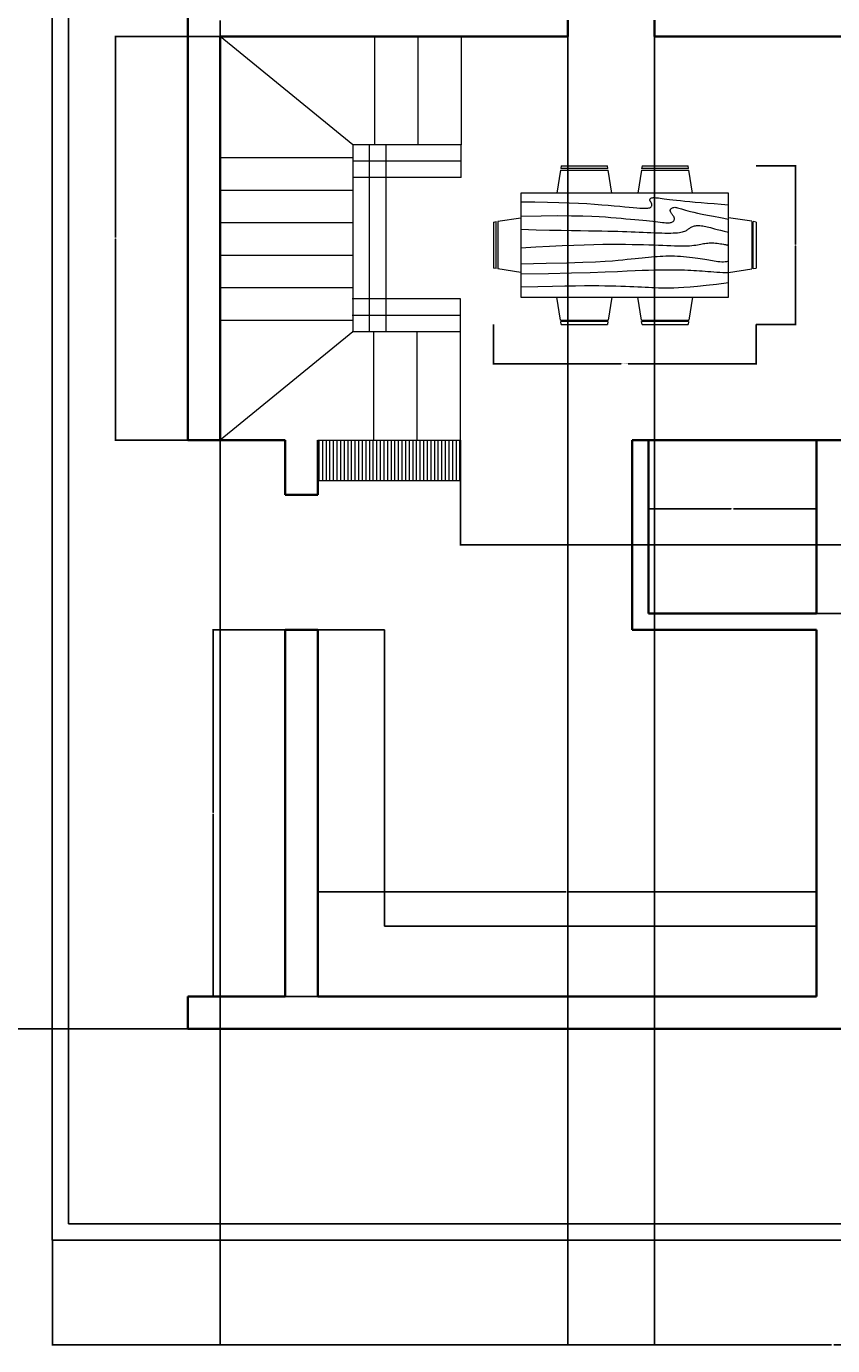
# Model space of a CAD drawing. Units: inches. Extents: x -1085 to 1941, y 1514 to 2348.
# Tile 2 of 9: x -836 to -613, y 1638 to 2003. Entities that reach past the tile are written whole.
import ezdxf

# ---------------------------------------------------------------- set-up
doc = ezdxf.new("R2010")
doc.units = ezdxf.units.IN
for name, color, linetype, lineweight in [('A-ANNO-DIMS', 2, 'Continuous', 18), ('A-FLOR-OTLN', 7, 'Continuous', 25), ('A-FLOR-PATT', 8, 'Continuous', 13), ('A-FLOR-STRS', 1, 'Continuous', 18), ('A-WALL', 7, 'Continuous', 35), ('C-PROP', 8, 'Continuous', 25), ('FOUNITR-URE', 2, 'Continuous', 18)]:
    doc.layers.add(name, color=color, linetype=linetype, lineweight=lineweight)
doc.styles.get("Standard").update_dxf_attribs({"font": 'arial.ttf'})
doc.dimstyles.get("Standard").update_dxf_attribs({"dimtxt": 0.18, "dimasz": 0.18, "dimexe": 0.18, "dimexo": 0.0625, "dimgap": 0.09, "dimtad": 0, "dimtih": 1, "dimtoh": 1, "dimdec": 4, "dimzin": 0, "dimdsep": 46, "dimtxsty": 'Standard', "dimcen": 0.09, "dimadec": 0, "dimazin": 0, "dimtfac": 1, "dimtdec": 4, "dimtofl": 0, "dimtmove": 0, "dimatfit": 3, "dimfxl": 1, "dimtolj": 1, "dimtzin": 0, "dimarcsym": 0})

# ---------------------------------------------------------------- blocks, each defined once
blk = doc.blocks.new('Dining Set - 36 x 72 in.')
for p, q in [((-22, 27.5), (-22.1562, 26.50042)), ((-22, 27.5), (-6, 27.5)), ((-5.8437, 26.49966), (-6, 27.5)), ((6, 27.5), (5.8438, 26.50042)), ((6, 27.5), (22, 27.5)), ((22.1563, 26.49966), (22, 27.5)), ((-22.2343, 26.00059), (-23.4847, 17.99762)), ((-22.2304, 26), (-5.7608, 26)), ((-5.8416, 26.5), (-22.1534, 26.5)), ((-4.5152, 17.99762), (-5.7655, 25.99926)), ((5.7657, 26.00059), (4.5153, 17.99762)), ((5.7696, 26), (22.2392, 26)), ((22.1584, 26.5), (5.8466, 26.5)), ((23.4848, 17.99762), (22.2345, 25.99926)), ((36, 18), (-36, 18)), ((-36, 18), (-36, -18)), ((36, -18), (36, 18)), ((-44.0006, 8.23428), (-35.9976, 9.48474)), ((44.0006, 8.23428), (35.9976, 9.48474)), ((-45.5, 8), (-44.5004, 8.15617)), ((-45.5, 8), (-45.5, -8)), ((-44.5, -8.15843), (-44.5, 8.15338)), ((-44, 8.23041), (-44, -8.23915)), ((44, 8.23041), (44, -8.23915)), ((44.5, -8.15843), (44.5, 8.15338)), ((45.5, 8), (44.5005, 8.15617)), ((45.5, 8), (45.5, -8)), ((-44.4997, -8.15631), (-45.5, -8)), ((-35.9976, -9.48476), (-43.9993, -8.2345)), ((35.9976, -9.48476), (43.9993, -8.2345)), ((44.4997, -8.15631), (45.5, -8)), ((-36, -18), (36, -18)), ((-22.2343, -26.0006), (-23.4847, -17.99762)), ((-4.5152, -17.99762), (-5.7655, -25.99928)), ((5.7657, -26.0006), (4.5153, -17.99762)), ((23.4848, -17.99762), (22.2345, -25.99928)), ((-22.2304, -26), (-5.7608, -26)), ((-22, -27.5), (-22.1562, -26.50044)), ((-5.8416, -26.5), (-22.1534, -26.5)), ((-5.8437, -26.49967), (-6, -27.5)), ((5.7696, -26), (22.2392, -26)), ((6, -27.5), (5.8438, -26.50044)), ((22.1584, -26.5), (5.8466, -26.5)), ((22.1563, -26.49967), (22, -27.5)), ((-22, -27.5), (-6, -27.5)), ((6, -27.5), (22, -27.5))]:
    blk.add_line(p, q)
for points in [[(-36, 15), (-31.1772, 14.97754), (-26.8079, 14.91406), (-22.8538, 14.81543), (-19.276, 14.6875), (-16.0362, 14.53613), (-13.0957, 14.36718), (-10.4159, 14.18652), (-7.9583, 14), (-5.6904, 13.81315), (-3.6035, 13.63021), (-1.6954, 13.45508), (0.0365, 13.29166), (1.5945, 13.14388), (2.9811, 13.01562), (4.1988, 12.9108), (5.25, 12.83333), (6.1393, 12.78613), (6.8802, 12.76823), (7.4883, 12.77767), (7.9792, 12.8125), (8.3685, 12.87077), (8.6719, 12.95052), (8.9049, 13.0498), (9.0833, 13.16666), (9.2205, 13.29899), (9.3216, 13.44401), (9.3895, 13.59879), (9.4271, 13.76041), (9.4373, 13.92594), (9.4232, 14.09245), (9.3875, 14.257), (9.3333, 14.41666), (9.2638, 14.56917), (9.1836, 14.71484), (9.0975, 14.85465), (9.0104, 14.98958), (8.9272, 15.1206), (8.8529, 15.2487), (8.7922, 15.37483), (8.75, 15.5), (8.7305, 15.62467), (8.7344, 15.74739), (8.7617, 15.86621), (8.8125, 15.97916), (8.8867, 16.08431), (8.9844, 16.17968), (9.1055, 16.26334), (9.25, 16.33333), (9.4189, 16.38802), (9.6172, 16.42708), (9.8506, 16.45052), (10.125, 16.45833), (10.4463, 16.45052), (10.8203, 16.42708), (11.2529, 16.38802), (11.75, 16.33333), (12.3184, 16.26318), (12.9694, 16.17838), (13.7151, 16.07991), (14.5677, 15.96875), (15.5395, 15.84586), (16.6426, 15.71224), (17.8893, 15.56884), (19.2917, 15.41666), (20.859, 15.25667), (22.5879, 15.08984), (24.4721, 14.91715), (26.5052, 14.73958), (28.6809, 14.5581), (30.9929, 14.3737), (33.4347, 14.18733), (36, 14)], [(-36, 10), (-28.9766, 10.14274), (-23.1725, 10.20442), (-18.4241, 10.19775), (-14.5677, 10.13541), (-11.4399, 10.03011), (-8.877, 9.89453), (-6.7154, 9.74137), (-4.7917, 9.58333), (-2.9698, 9.43082), (-1.2246, 9.28515), (0.4415, 9.14534), (2.026, 9.01041), (3.5266, 8.87939), (4.9408, 8.7513), (6.266, 8.62516), (7.5, 8.5), (8.6411, 8.37549), (9.6914, 8.2539), (10.6538, 8.13818), (11.5312, 8.03125), (12.3267, 7.93603), (13.043, 7.85547), (13.6831, 7.79248), (14.25, 7.75), (14.7471, 7.7303), (15.1797, 7.73307), (15.5537, 7.75732), (15.875, 7.80208), (16.1494, 7.86637), (16.3828, 7.94922), (16.5811, 8.04964), (16.75, 8.16666), (16.8944, 8.29915), (17.0143, 8.44531), (17.1089, 8.60319), (17.1771, 8.77083), (17.218, 8.94629), (17.2305, 9.1276), (17.2137, 9.31282), (17.1667, 9.5), (17.0895, 9.6875), (16.987, 9.875), (16.8649, 10.0625), (16.7292, 10.25), (16.5856, 10.4375), (16.4401, 10.625), (16.2985, 10.8125), (16.1667, 11), (16.05, 11.18733), (15.9518, 11.3737), (15.8752, 11.5581), (15.8229, 11.73958), (15.798, 11.91715), (15.8034, 12.08984), (15.842, 12.25667), (15.9167, 12.41666), (16.0295, 12.56836), (16.1784, 12.70833), (16.3605, 12.83268), (16.5729, 12.9375), (16.8127, 13.01888), (17.0768, 13.07291), (17.3625, 13.0957), (17.6667, 13.08333), (17.9894, 13.03312), (18.3418, 12.94726), (18.7382, 12.82918), (19.1927, 12.68229), (19.7195, 12.51001), (20.3327, 12.31575), (21.0465, 12.10294), (21.875, 11.875), (22.8357, 11.63354), (23.959, 11.37304), (25.2786, 11.08618), (26.8282, 10.76562), (28.6414, 10.40405), (30.752, 9.99414), (33.1936, 9.52856), (36, 9)], [(-36, 5.5), (-30.7157, 5.3348), (-26.069, 5.20963), (-21.9946, 5.11767), (-18.4271, 5.05208), (-15.3009, 5.00602), (-12.5508, 4.97265), (-10.1112, 4.94515), (-7.9167, 4.91666), (-5.909, 4.88167), (-4.0586, 4.83984), (-2.3429, 4.79215), (-0.7396, 4.73958), (0.7739, 4.6831), (2.22, 4.6237), (3.6213, 4.56233), (5, 4.5), (6.373, 4.43782), (7.7344, 4.3776), (9.0723, 4.32129), (10.375, 4.27083), (11.6309, 4.22819), (12.8281, 4.19531), (13.9551, 4.17415), (15, 4.16666), (15.954, 4.17448), (16.819, 4.19791), (17.6001, 4.23698), (18.3021, 4.29166), (18.9299, 4.36198), (19.4883, 4.44791), (19.9823, 4.54948), (20.4167, 4.66666), (20.7969, 4.79899), (21.1302, 4.94401), (21.4245, 5.09879), (21.6875, 5.26041), (21.9271, 5.42594), (22.1511, 5.59245), (22.3672, 5.757), (22.5834, 5.91666), (22.8065, 6.06868), (23.0404, 6.21093), (23.2879, 6.34147), (23.5521, 6.45833), (23.8358, 6.55957), (24.142, 6.64323), (24.4735, 6.70735), (24.8334, 6.75), (25.2235, 6.76969), (25.642, 6.76692), (26.0858, 6.74267), (26.5521, 6.69791), (27.0379, 6.63362), (27.5404, 6.55078), (28.0565, 6.45036), (28.5834, 6.33333), (29.1242, 6.19987), (29.7071, 6.04687), (30.3661, 5.87044), (31.1354, 5.66666), (32.0493, 5.43164), (33.142, 5.16146), (34.4475, 4.85221), (36, 4.5)], [(-36, -1), (-30.7915, -0.6591), (-26.0195, -0.38216), (-21.6519, -0.16284), (-17.6563, 0.00521), (-14.0005, 0.12833), (-10.6523, 0.21289), (-7.5796, 0.26522), (-4.75, 0.29166), (-2.134, 0.29793), (0.2878, 0.28711), (2.5317, 0.26163), (4.6146, 0.22396), (6.5529, 0.17651), (8.3633, 0.12174), (10.0623, 0.06209), (11.6667, 0), (13.1899, -0.06201), (14.6341, -0.1211), (15.9982, -0.17432), (17.2813, -0.21875), (18.4823, -0.25147), (19.6003, -0.26953), (20.6343, -0.27002), (21.5834, -0.25), (22.4481, -0.20768), (23.2357, -0.14584), (23.9549, -0.06836), (24.6146, 0.02083), (25.2235, 0.11784), (25.7904, 0.21875), (26.3241, 0.31966), (26.8334, 0.41666), (27.3265, 0.50618), (27.8099, 0.58593), (28.2894, 0.65397), (28.7709, 0.70833), (29.2601, 0.74707), (29.763, 0.76823), (30.2855, 0.76985), (30.8334, 0.75), (31.4088, 0.70784), (31.9994, 0.64713), (32.589, 0.57275), (33.1615, 0.48958), (33.7008, 0.4025), (34.1908, 0.3164), (34.6153, 0.23616), (34.9584, 0.16666), (35.2099, 0.11165), (35.3848, 0.07031), (35.504, 0.04069), (35.5886, 0.02083), (35.6594, 0.00879), (35.7377, 0.0026), (35.8442, 0.00032), (36, 0)], [(-36, -6.5), (-27.1843, -6.31267), (-20.084, -6.1263), (-14.469, -5.9419), (-10.1094, -5.76042), (-6.7752, -5.58285), (-4.2363, -5.41016), (-2.2629, -5.24333), (-0.625, -5.08334), (0.8708, -4.93099), (2.2715, -4.78646), (3.5872, -4.64974), (4.8281, -4.52084), (6.0046, -4.39974), (7.127, -4.28646), (8.2053, -4.18099), (9.25, -4.08334), (10.2705, -3.99382), (11.2734, -3.91407), (12.2647, -3.84603), (13.25, -3.79167), (14.2354, -3.75293), (15.2266, -3.73177), (16.2295, -3.73015), (17.25, -3.75), (18.2912, -3.79248), (19.3451, -3.85547), (20.4009, -3.93604), (21.4479, -4.03125), (22.4754, -4.13819), (23.4727, -4.25391), (24.4289, -4.37549), (25.3334, -4.5), (26.1785, -4.62492), (26.9694, -4.74935), (27.7145, -4.87281), (28.4219, -4.99479), (29.1, -5.11483), (29.7572, -5.23242), (30.4016, -5.34709), (31.0417, -5.45834), (31.6837, -5.56437), (32.3262, -5.65821), (32.9658, -5.73153), (33.599, -5.77604), (34.2224, -5.78345), (34.8327, -5.74545), (35.4264, -5.65373), (36, -5.5)], [(-36, -10), (-26.4022, -9.81299), (-18.4675, -9.62891), (-11.9839, -9.45069), (-6.7396, -9.28125), (-2.5226, -9.12354), (0.8789, -8.98047), (3.6769, -8.85498), (6.0833, -8.75), (8.2767, -8.66765), (10.3021, -8.60677), (12.1712, -8.56543), (13.8958, -8.54167), (15.4876, -8.53353), (16.9583, -8.53907), (18.3197, -8.55632), (19.5834, -8.58334), (20.7616, -8.61841), (21.8685, -8.66081), (22.9188, -8.71004), (23.9271, -8.76563), (24.9081, -8.82707), (25.8763, -8.89388), (26.8465, -8.96558), (27.8334, -9.04167), (28.8474, -9.12118), (29.8828, -9.20117), (30.93, -9.27824), (31.9792, -9.34896), (33.0205, -9.40991), (34.0443, -9.45768), (35.0407, -9.48885), (36, -9.5)], [(-36, -14.5), (-30.0881, -14.33513), (-25.0332, -14.21224), (-20.7312, -14.12647), (-17.0781, -14.07292), (-13.97, -14.04671), (-11.3027, -14.04297), (-8.9724, -14.05681), (-6.875, -14.08334), (-4.9224, -14.11833), (-3.0905, -14.16016), (-1.3709, -14.20785), (0.2448, -14.26042), (1.7647, -14.3169), (3.1973, -14.3763), (4.5507, -14.43767), (5.8333, -14.5), (7.0554, -14.5621), (8.235, -14.62175), (9.3922, -14.67652), (10.5469, -14.72396), (11.7192, -14.76164), (12.929, -14.78711), (14.1965, -14.79794), (15.5417, -14.79167), (16.9933, -14.76424), (18.6152, -14.70508), (20.4804, -14.60197), (22.6615, -14.44271), (25.2312, -14.21509), (28.2624, -13.9069), (31.8277, -13.50594), (36, -13)]]:
    blk.add_lwpolyline(points)
blk = doc.blocks.new('*D62')
at = {"layer": 'A-ANNO-DIMS', "color": 0, "lineweight": -2, "transparency": 16777216}
for p, q in [((-706.5, 1920.37), (-706.5, 1909.35)), ((-633.81, 1920.37), (-633.81, 1909.35)), ((-706.32, 1909.53), (-671.12, 1909.53)), ((-633.99, 1909.53), (-669.18, 1909.53))]:
    blk.add_line(p, q, dxfattribs=at)
at = {"layer": 'A-ANNO-DIMS', "color": 0, "transparency": 16777216}
for points in [[(-706.32, 1909.56), (-706.32, 1909.5), (-706.5, 1909.53)], [(-633.99, 1909.56), (-633.99, 1909.5), (-633.81, 1909.53)]]:
    blk.add_solid(points, dxfattribs=at)
at = {"layer": 'Defpoints', "color": 0, "transparency": 16777216}
for p in [(-706.5, 1920.43), (-633.81, 1920.43), (-633.81, 1909.53)]:
    blk.add_point(p, dxfattribs=at)
at = {"layer": 'A-ANNO-DIMS', "color": 0, "transparency": 16777216, "insert": (-670.15, 1909.53), "char_height": 0.18, "attachment_point": 5}
blk.add_mtext('\\A1;DINING SET 73', dxfattribs=at)
blk = doc.blocks.new('*D63')
at = {"layer": 'A-ANNO-DIMS', "color": 0, "lineweight": -2, "transparency": 16777216}
for p, q in [((-633.75, 1964.36), (-622.73, 1964.36)), ((-622.91, 1964.18), (-622.91, 1942.58)), ((-622.91, 1920.61), (-622.91, 1942.22)), ((-633.75, 1920.43), (-622.73, 1920.43))]:
    blk.add_line(p, q, dxfattribs=at)
at = {"layer": 'A-ANNO-DIMS', "color": 0, "transparency": 16777216}
for points in [[(-622.94, 1964.18), (-622.88, 1964.18), (-622.91, 1964.36)], [(-622.94, 1920.61), (-622.88, 1920.61), (-622.91, 1920.43)]]:
    blk.add_solid(points, dxfattribs=at)
at = {"layer": 'Defpoints', "color": 0, "transparency": 16777216}
for p in [(-633.81, 1964.36), (-622.91, 1964.36), (-633.81, 1920.43)]:
    blk.add_point(p, dxfattribs=at)
at = {"layer": 'A-ANNO-DIMS', "color": 0, "transparency": 16777216, "insert": (-622.91, 1942.4), "char_height": 0.18, "attachment_point": 5}
blk.add_mtext('\\A1;44', dxfattribs=at)
blk = doc.blocks.new('*D94')
at = {"layer": 'A-ANNO-DIMS', "color": 0, "lineweight": -2, "transparency": 16777216}
for p, q in [((-828.6, 1666.82), (-828.6, 1637.7)), ((-396.6, 1666.82), (-396.6, 1637.7)), ((-828.42, 1637.88), (-612.89, 1637.88)), ((-396.78, 1637.88), (-612.31, 1637.88))]:
    blk.add_line(p, q, dxfattribs=at)
at = {"layer": 'A-ANNO-DIMS', "color": 0, "transparency": 16777216}
for points in [[(-828.42, 1637.91), (-828.42, 1637.85), (-828.6, 1637.88)], [(-396.78, 1637.91), (-396.78, 1637.85), (-396.6, 1637.88)]]:
    blk.add_solid(points, dxfattribs=at)
at = {"layer": 'Defpoints', "color": 0, "transparency": 16777216}
for p in [(-828.6, 1666.88), (-396.6, 1666.88), (-396.6, 1637.88)]:
    blk.add_point(p, dxfattribs=at)
at = {"layer": 'A-ANNO-DIMS', "color": 0, "transparency": 16777216, "insert": (-612.6, 1637.88), "char_height": 0.18, "attachment_point": 5}
blk.add_mtext('\\A1;432', dxfattribs=at)
blk = doc.blocks.new('*D97')
at = {"layer": 'A-ANNO-DIMS', "color": 0, "lineweight": -2, "transparency": 16777216}
for p, q in [((-791.17, 2205.38), (-857.78, 2205.38)), ((-857.6, 2205.2), (-857.6, 1965.57)), ((-857.6, 1725.56), (-857.6, 1965.2)), ((-791.17, 1725.38), (-857.78, 1725.38))]:
    blk.add_line(p, q, dxfattribs=at)
at = {"layer": 'A-ANNO-DIMS', "color": 0, "transparency": 16777216}
for points in [[(-857.63, 2205.2), (-857.57, 2205.2), (-857.6, 2205.38)], [(-857.63, 1725.56), (-857.57, 1725.56), (-857.6, 1725.38)]]:
    blk.add_solid(points, dxfattribs=at)
at = {"layer": 'Defpoints', "color": 0, "transparency": 16777216}
for p in [(-791.1, 2205.38), (-857.6, 1725.38), (-791.1, 1725.38)]:
    blk.add_point(p, dxfattribs=at)
at = {"layer": 'A-ANNO-DIMS', "color": 0, "transparency": 16777216, "insert": (-857.6, 1965.38), "char_height": 0.18, "attachment_point": 5}
blk.add_mtext('\\A1;480', dxfattribs=at)
blk = doc.blocks.new('*D106')
at = {"layer": 'A-ANNO-DIMS', "color": 0, "lineweight": -2, "transparency": 16777216}
for p, q in [((-685.88, 2004.62), (-685.88, 1637.7)), ((-661.88, 2004.62), (-661.88, 1637.7)), ((-685.7, 1637.88), (-674.1, 1637.88)), ((-662.06, 1637.88), (-673.66, 1637.88))]:
    blk.add_line(p, q, dxfattribs=at)
at = {"layer": 'A-ANNO-DIMS', "color": 0, "transparency": 16777216}
for points in [[(-685.7, 1637.91), (-685.7, 1637.85), (-685.88, 1637.88)], [(-662.06, 1637.91), (-662.06, 1637.85), (-661.88, 1637.88)]]:
    blk.add_solid(points, dxfattribs=at)
at = {"layer": 'Defpoints', "color": 0, "transparency": 16777216}
for p in [(-685.88, 2004.68), (-661.88, 2004.68), (-685.88, 1637.88)]:
    blk.add_point(p, dxfattribs=at)
at = {"layer": 'A-ANNO-DIMS', "color": 0, "transparency": 16777216, "insert": (-673.88, 1637.88), "char_height": 0.18, "attachment_point": 5}
blk.add_mtext('\\A1;24', dxfattribs=at)
blk = doc.blocks.new('*D107')
at = {"layer": 'A-ANNO-DIMS', "color": 0, "lineweight": -2, "transparency": 16777216}
for p, q in [((-782.1, 2004.62), (-782.1, 1637.7)), ((-685.88, 2004.62), (-685.88, 1637.7)), ((-781.92, 1637.88), (-734.38, 1637.88)), ((-686.06, 1637.88), (-733.6, 1637.88))]:
    blk.add_line(p, q, dxfattribs=at)
at = {"layer": 'A-ANNO-DIMS', "color": 0, "transparency": 16777216}
for points in [[(-781.92, 1637.91), (-781.92, 1637.85), (-782.1, 1637.88)], [(-686.06, 1637.91), (-686.06, 1637.85), (-685.88, 1637.88)]]:
    blk.add_solid(points, dxfattribs=at)
at = {"layer": 'Defpoints', "color": 0, "transparency": 16777216}
for p in [(-782.1, 2004.68), (-685.88, 2004.68), (-782.1, 1637.88)]:
    blk.add_point(p, dxfattribs=at)
at = {"layer": 'A-ANNO-DIMS', "color": 0, "transparency": 16777216, "insert": (-733.99, 1637.88), "char_height": 0.18, "attachment_point": 5}
blk.add_mtext('\\A1;96.23', dxfattribs=at)
blk = doc.blocks.new('*D111')
at = {"layer": 'A-ANNO-DIMS', "color": 0, "lineweight": -2, "transparency": 16777216}
for p, q in [((-782.17, 2000.18), (-811.28, 2000.18)), ((-811.1, 2000), (-811.1, 1944.46)), ((-811.1, 1888.56), (-811.1, 1944.1)), ((-782.17, 1888.38), (-811.28, 1888.38))]:
    blk.add_line(p, q, dxfattribs=at)
at = {"layer": 'A-ANNO-DIMS', "color": 0, "transparency": 16777216}
for points in [[(-811.13, 2000), (-811.07, 2000), (-811.1, 2000.18)], [(-811.13, 1888.56), (-811.07, 1888.56), (-811.1, 1888.38)]]:
    blk.add_solid(points, dxfattribs=at)
at = {"layer": 'Defpoints', "color": 0, "transparency": 16777216}
for p in [(-811.1, 2000.18), (-782.1, 2000.18), (-782.1, 1888.38)]:
    blk.add_point(p, dxfattribs=at)
at = {"layer": 'A-ANNO-DIMS', "color": 0, "transparency": 16777216, "insert": (-811.1, 1944.28), "char_height": 0.18, "attachment_point": 5}
blk.add_mtext('\\A1;111.8', dxfattribs=at)
blk = doc.blocks.new('*D112')
at = {"layer": 'A-ANNO-DIMS', "color": 0, "lineweight": -2, "transparency": 16777216}
for p, q in [((-715.62, 1888.32), (-715.62, 1859.2)), ((-446.1, 1888.32), (-446.1, 1859.2)), ((-715.44, 1859.38), (-581.26, 1859.38)), ((-446.28, 1859.38), (-580.47, 1859.38))]:
    blk.add_line(p, q, dxfattribs=at)
at = {"layer": 'A-ANNO-DIMS', "color": 0, "transparency": 16777216}
for points in [[(-715.44, 1859.41), (-715.44, 1859.35), (-715.62, 1859.38)], [(-446.28, 1859.41), (-446.28, 1859.35), (-446.1, 1859.38)]]:
    blk.add_solid(points, dxfattribs=at)
at = {"layer": 'Defpoints', "color": 0, "transparency": 16777216}
for p in [(-715.62, 1888.38), (-446.1, 1888.38), (-715.62, 1859.38)]:
    blk.add_point(p, dxfattribs=at)
at = {"layer": 'A-ANNO-DIMS', "color": 0, "transparency": 16777216, "insert": (-580.86, 1859.38), "char_height": 0.18, "attachment_point": 5}
blk.add_mtext('\\A1;269.5', dxfattribs=at)
blk = doc.blocks.new('*D115')
at = {"layer": 'A-ANNO-DIMS', "color": 0, "lineweight": -2, "transparency": 16777216}
for p, q in [((-755.1, 1734.45), (-755.1, 1763.56)), ((-754.92, 1763.38), (-686.38, 1763.38)), ((-617.28, 1763.38), (-685.82, 1763.38)), ((-617.1, 1734.45), (-617.1, 1763.56))]:
    blk.add_line(p, q, dxfattribs=at)
at = {"layer": 'A-ANNO-DIMS', "color": 0, "transparency": 16777216}
for points in [[(-754.92, 1763.41), (-754.92, 1763.35), (-755.1, 1763.38)], [(-617.28, 1763.41), (-617.28, 1763.35), (-617.1, 1763.38)]]:
    blk.add_solid(points, dxfattribs=at)
at = {"layer": 'Defpoints', "color": 0, "transparency": 16777216}
for p in [(-617.1, 1763.38), (-755.1, 1734.38), (-617.1, 1734.38)]:
    blk.add_point(p, dxfattribs=at)
at = {"layer": 'A-ANNO-DIMS', "color": 0, "transparency": 16777216, "insert": (-686.1, 1763.38), "char_height": 0.18, "attachment_point": 5}
blk.add_mtext('\\A1;138', dxfattribs=at)
blk = doc.blocks.new('*D116')
at = {"layer": 'A-ANNO-DIMS', "color": 0, "lineweight": -2, "transparency": 16777216}
for p, q in [((-755.17, 1835.88), (-784.28, 1835.88)), ((-784.1, 1835.7), (-784.1, 1785.32)), ((-784.1, 1734.56), (-784.1, 1784.95)), ((-755.17, 1734.38), (-784.28, 1734.38))]:
    blk.add_line(p, q, dxfattribs=at)
at = {"layer": 'A-ANNO-DIMS', "color": 0, "transparency": 16777216}
for points in [[(-784.13, 1835.7), (-784.07, 1835.7), (-784.1, 1835.88)], [(-784.13, 1734.56), (-784.07, 1734.56), (-784.1, 1734.38)]]:
    blk.add_solid(points, dxfattribs=at)
at = {"layer": 'Defpoints', "color": 0, "transparency": 16777216}
for p in [(-784.1, 1835.88), (-755.1, 1835.88), (-755.1, 1734.38)]:
    blk.add_point(p, dxfattribs=at)
at = {"layer": 'A-ANNO-DIMS', "color": 0, "transparency": 16777216, "insert": (-784.1, 1785.13), "char_height": 0.18, "attachment_point": 5}
blk.add_mtext('\\A1;101.5', dxfattribs=at)
blk = doc.blocks.new('*D117')
at = {"layer": 'A-ANNO-DIMS', "color": 0, "lineweight": -2, "transparency": 16777216}
for p, q in [((-663.6, 1840.45), (-663.6, 1869.56)), ((-663.42, 1869.38), (-640.68, 1869.38)), ((-617.28, 1869.38), (-640.03, 1869.38)), ((-617.1, 1840.45), (-617.1, 1869.56))]:
    blk.add_line(p, q, dxfattribs=at)
at = {"layer": 'A-ANNO-DIMS', "color": 0, "transparency": 16777216}
for points in [[(-663.42, 1869.41), (-663.42, 1869.35), (-663.6, 1869.38)], [(-617.28, 1869.41), (-617.28, 1869.35), (-617.1, 1869.38)]]:
    blk.add_solid(points, dxfattribs=at)
at = {"layer": 'Defpoints', "color": 0, "transparency": 16777216}
for p in [(-617.1, 1869.38), (-663.6, 1840.38), (-617.1, 1840.38)]:
    blk.add_point(p, dxfattribs=at)
at = {"layer": 'A-ANNO-DIMS', "color": 0, "transparency": 16777216, "insert": (-640.35, 1869.38), "char_height": 0.18, "attachment_point": 5}
blk.add_mtext('\\A1;46.5', dxfattribs=at)
blk = doc.blocks.new('*D118')
at = {"layer": 'A-ANNO-DIMS', "color": 0, "lineweight": -2, "transparency": 16777216}
for p, q in [((-617.04, 1888.38), (-587.92, 1888.38)), ((-588.1, 1888.2), (-588.1, 1864.57)), ((-588.1, 1840.56), (-588.1, 1864.2)), ((-617.04, 1840.38), (-587.92, 1840.38))]:
    blk.add_line(p, q, dxfattribs=at)
at = {"layer": 'A-ANNO-DIMS', "color": 0, "transparency": 16777216}
for points in [[(-588.13, 1888.2), (-588.07, 1888.2), (-588.1, 1888.38)], [(-588.13, 1840.56), (-588.07, 1840.56), (-588.1, 1840.38)]]:
    blk.add_solid(points, dxfattribs=at)
at = {"layer": 'Defpoints', "color": 0, "transparency": 16777216}
for p in [(-617.1, 1888.38), (-617.1, 1840.38), (-588.1, 1840.38)]:
    blk.add_point(p, dxfattribs=at)
at = {"layer": 'A-ANNO-DIMS', "color": 0, "transparency": 16777216, "insert": (-588.1, 1864.38), "char_height": 0.18, "attachment_point": 5}
blk.add_mtext('\\A1;48', dxfattribs=at)

msp = doc.modelspace()

# ---------------------------------------------------------------- hatches: boundary and pattern name
at = {"layer": 'A-FLOR-PATT'}
h = msp.add_hatch(dxfattribs=at)
h.set_pattern_fill('ANSI31', color=256, scale=0.314961, angle=45, style=0)
h.set_pattern_definition([(90, (-2122.7521, 0), (-1, 0), [])])
h.paths.add_polyline_path([(-755.1032, 1877.156), (-715.6221, 1877.156), (-715.6221, 1888.3835), (-755.1032, 1888.3835)])

# ---------------------------------------------------------------- linework, layer by layer
at = {"layer": 'A-FLOR-OTLN'}
for p, q in [((-755.1032, 1835.8835), (-736.634, 1835.8835)), ((-736.634, 1835.8835), (-736.634, 1753.8429)), ((-736.634, 1753.8429), (-617.1032, 1753.8429))]:
    msp.add_line(p, q, dxfattribs=at)
at = {"layer": 'A-FLOR-STRS'}
for p, q in [((-745.409, 1970.1777), (-782.1032, 2000.1777)), ((-739.409, 2000.1777), (-739.409, 1970.1777)), ((-727.409, 2000.1777), (-727.409, 1970.1777)), ((-715.409, 2000.1777), (-715.409, 1970.1777)), ((-715.409, 1970.1777), (-745.409, 1970.1777)), ((-745.409, 1970.1777), (-745.409, 1918.3835)), ((-740.854, 1970.1777), (-740.854, 1918.3835)), ((-736.2989, 1970.1777), (-736.2989, 1918.3835)), ((-715.409, 1961.0676), (-715.409, 1970.1777)), ((-745.409, 1966.5562), (-782.1032, 1966.5562)), ((-715.409, 1965.6226), (-745.409, 1965.6226)), ((-715.409, 1961.0676), (-745.409, 1961.0676)), ((-745.409, 1957.5562), (-782.1032, 1957.5562)), ((-745.409, 1948.5562), (-782.1032, 1948.5562)), ((-745.409, 1939.5562), (-782.1032, 1939.5562)), ((-745.409, 1930.5562), (-782.1032, 1930.5562)), ((-715.6221, 1927.4936), (-745.6221, 1927.4936)), ((-715.6221, 1918.3835), (-715.6221, 1927.4936)), ((-745.409, 1921.5562), (-782.1032, 1921.5562)), ((-715.6221, 1922.9386), (-745.6221, 1922.9386)), ((-745.409, 1918.3835), (-782.1032, 1888.3835)), ((-715.6221, 1918.3835), (-745.6221, 1918.3835)), ((-739.6221, 1888.3835), (-739.6221, 1918.3835)), ((-727.6221, 1888.3835), (-727.6221, 1918.3835)), ((-715.6221, 1888.3835), (-715.6221, 1918.3835)), ((-755.1032, 1888.3835), (-715.6221, 1888.3835)), ((-715.6221, 1888.3835), (-715.6221, 1877.156)), ((-715.6221, 1877.156), (-755.1032, 1877.156))]:
    msp.add_line(p, q, dxfattribs=at)
at = {"layer": 'A-WALL'}
for p, q in [((-791.1032, 1888.3835), (-791.1032, 2205.3835)), ((-685.8764, 2000.1777), (-685.8764, 2004.6777)), ((-661.8764, 2004.6777), (-661.8764, 2000.1777)), ((-782.1032, 1888.3835), (-782.1032, 2000.1777)), ((-685.8764, 2000.1777), (-782.1032, 2000.1777)), ((-645.6032, 2000.1777), (-661.8764, 2000.1777)), ((-645.6032, 2000.1777), (-591.6032, 2000.1777)), ((-764.1032, 1888.3835), (-791.1032, 1888.3835)), ((-764.1032, 1873.2355), (-764.1032, 1888.3835)), ((-755.1032, 1873.2355), (-755.1032, 1888.3835)), ((-617.1032, 1888.3835), (-668.1032, 1888.3835)), ((-668.1032, 1888.3835), (-668.1032, 1835.8835)), ((-663.6032, 1888.3835), (-663.6032, 1840.3835)), ((-617.1032, 1888.3835), (-496.941, 1888.3835)), ((-617.1032, 1840.3835), (-617.1032, 1888.3835)), ((-755.1032, 1873.2355), (-764.1032, 1873.2355)), ((-663.6032, 1840.3835), (-617.1032, 1840.3835)), ((-764.1032, 1835.8835), (-764.1032, 1743.9418)), ((-764.1032, 1743.9418), (-764.1032, 1835.8835)), ((-755.1032, 1835.8835), (-764.1032, 1835.8835)), ((-755.1032, 1743.9418), (-755.1032, 1835.8835)), ((-668.1032, 1835.8835), (-617.1032, 1835.8835)), ((-617.1032, 1734.3835), (-617.1032, 1835.8835)), ((-617.1032, 1835.8835), (-617.1032, 1734.3835)), ((-764.1032, 1743.9418), (-764.1032, 1734.3835)), ((-755.1032, 1743.9418), (-755.1032, 1743.9418)), ((-755.1032, 1743.9418), (-755.1032, 1739.7262)), ((-755.1032, 1739.7262), (-755.1032, 1739.7262)), ((-755.1032, 1739.7262), (-755.1032, 1734.3835)), ((-791.1032, 1725.3835), (-791.1032, 1734.3835)), ((-764.1032, 1734.3835), (-791.1032, 1734.3835)), ((-617.1032, 1734.3835), (-755.1032, 1734.3835)), ((-608.1032, 1725.3835), (-791.1032, 1725.3835))]:
    msp.add_line(p, q, dxfattribs=at)
at = {"layer": 'C-PROP'}
for p, q in [((-828.6032, 1666.8835), (-828.6032, 2242.8835)), ((-824.1032, 1671.3835), (-824.1032, 2238.3835)), ((-401.1032, 1671.3835), (-824.1032, 1671.3835)), ((-396.6032, 1666.8835), (-828.6032, 1666.8835))]:
    msp.add_line(p, q, dxfattribs=at)

# ---------------------------------------------------------------- block references
at = {"layer": 'FOUNITR-URE', "xscale": 0.7987481626501499, "yscale": 0.7987481626501499, "zscale": 0.7987481626501499}
msp.add_blockref('Dining Set - 36 x 72 in.', (-670.152, 1942.3975), dxfattribs=at)

# ---------------------------------------------------------------- dimensions: what is measured, and where the dimension line sits
at = {"layer": 'A-ANNO-DIMS'}
for base, p1, p2, angle, override, picture, middle in [((-857.6032, 1725.3835), (-791.1032, 2205.3835), (-791.1032, 1725.3835), 90, {"dimdec": 0, "dimlfac": 1, "dimrnd": 0, "dimzin": 0, "dimdsep": 46, "dimlunit": 2}, '*D97', (-857.6032, 1965.3835)), ((-811.1032, 2000.1777), (-782.1032, 1888.3835), (-782.1032, 2000.1777), 90, {"dimdec": 1, "dimlfac": 1, "dimrnd": 0, "dimzin": 0, "dimdsep": 46, "dimlunit": 2}, '*D111', (-811.1032, 1944.2806)), ((-622.906, 1964.3631), (-633.809, 1920.432), (-633.809, 1964.3631), 90, {"dimdec": 0, "dimlfac": 1, "dimrnd": 0, "dimzin": 0, "dimdsep": 46, "dimlunit": 2}, '*D63', (-622.906, 1942.3975)), ((-715.6221, 1859.3835), (-446.1032, 1888.3835), (-715.6221, 1888.3835), 180, {"dimdec": 1, "dimlfac": 1, "dimrnd": 0, "dimzin": 0, "dimdsep": 46, "dimlunit": 2}, '*D112', (-580.8627, 1859.3835)), ((-588.1032, 1840.3835), (-617.1032, 1888.3835), (-617.1032, 1840.3835), 270, {"dimdec": 0, "dimlfac": 1, "dimrnd": 0, "dimzin": 0, "dimdsep": 46, "dimlunit": 2}, '*D118', (-588.1032, 1864.3835)), ((-784.1032, 1835.8835), (-755.1032, 1734.3835), (-755.1032, 1835.8835), 90, {"dimdec": 1, "dimlfac": 1, "dimrnd": 0, "dimzin": 0, "dimdsep": 46, "dimlunit": 2}, '*D116', (-784.1032, 1785.1335))]:
    dim = msp.add_linear_dim(base=base, p1=p1, p2=p2, angle=angle, dimstyle='Standard', override=override, dxfattribs=at)
    dim.commit()
    dim.dimension.update_dxf_attribs({"geometry": picture, "text_midpoint": middle})
for base, p1, p2, override, picture, middle in [((-782.1032, 1637.8835), (-685.8764, 2004.6777), (-782.1032, 2004.6777), {"dimdec": 2, "dimlfac": 1, "dimrnd": 0, "dimzin": 0, "dimdsep": 46, "dimlunit": 2}, '*D107', (-733.9898, 1637.8835)), ((-685.8764, 1637.8835), (-661.8764, 2004.6777), (-685.8764, 2004.6777), {"dimdec": 0, "dimlfac": 1, "dimrnd": 0, "dimzin": 0, "dimdsep": 46, "dimlunit": 2}, '*D106', (-673.8764, 1637.8835)), ((-617.1032, 1869.3835), (-663.6032, 1840.3835), (-617.1032, 1840.3835), {"dimdec": 1, "dimlfac": 1, "dimrnd": 0, "dimzin": 0, "dimdsep": 46, "dimlunit": 2}, '*D117', (-640.3532, 1869.3835)), ((-617.1032, 1763.3835), (-755.1032, 1734.3835), (-617.1032, 1734.3835), {"dimdec": 0, "dimlfac": 1, "dimrnd": 0, "dimzin": 0, "dimdsep": 46, "dimlunit": 2}, '*D115', (-686.1032, 1763.3835)), ((-396.6032, 1637.8835), (-828.6032, 1666.8835), (-396.6032, 1666.8835), {"dimdec": 0, "dimlfac": 1, "dimrnd": 0, "dimzin": 0, "dimdsep": 46, "dimlunit": 2}, '*D94', (-612.6032, 1637.8835))]:
    dim = msp.add_linear_dim(base=base, p1=p1, p2=p2, dimstyle='Standard', override=override, dxfattribs=at)
    dim.commit()
    dim.dimension.update_dxf_attribs({"geometry": picture, "text_midpoint": middle})
dim = msp.add_linear_dim(base=(-633.809, 1909.529), p1=(-706.495, 1920.432), p2=(-633.809, 1920.432), text='DINING SET <>', dimstyle='Standard', override={"dimdec": 0, "dimlfac": 1, "dimrnd": 0, "dimzin": 0, "dimdsep": 46, "dimlunit": 2}, dxfattribs=at)
dim.commit()
dim.dimension.update_dxf_attribs({"geometry": '*D62', "text_midpoint": (-670.152, 1909.529)})

doc.saveas('drawing.dxf')
